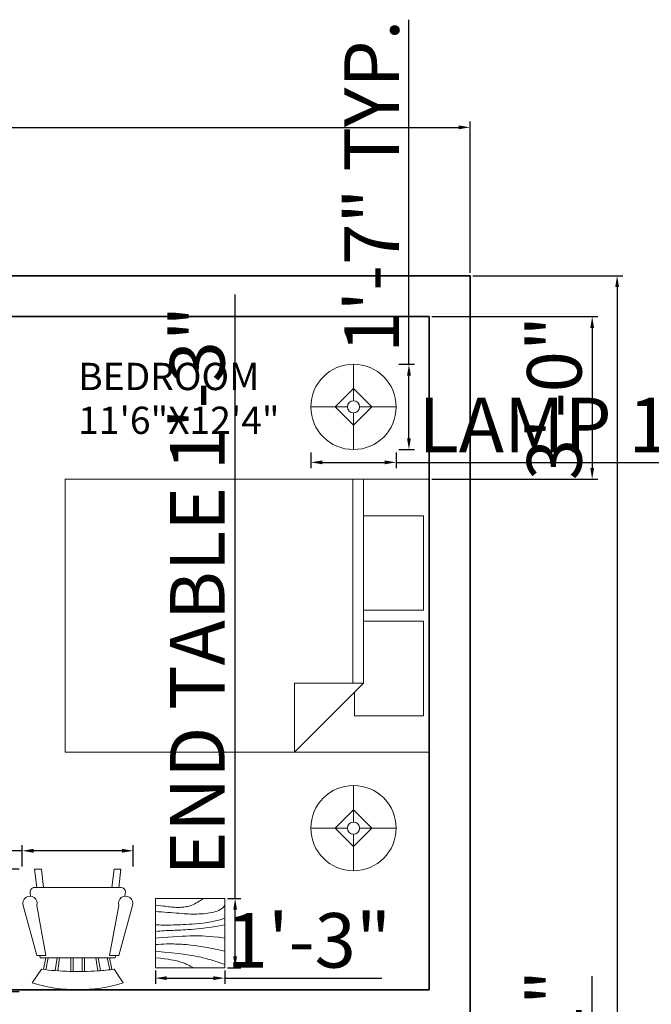
# Model space of a CAD drawing. Units: inches. Extents: x 2446 to 3341, y 462 to 1195.
# Tile 4 of 6: x 2746 to 2884, y 888 to 1104. Entities that reach past the tile are written whole.
import ezdxf

# ---------------------------------------------------------------- set-up
doc = ezdxf.new("R2010")
doc.units = ezdxf.units.IN
for name, color, linetype, lineweight in [('A-ANNO-DIMS', 2, 'Continuous', 18), ('A-AREA-IDEN', 7, 'Continuous', 18), ('A-FURN', 8, 'Continuous', 18), ('A-WALL', 7, 'Continuous', 35), ('C-PROP', 7, 'Continuous', 35)]:
    doc.layers.add(name, color=color, linetype=linetype, lineweight=lineweight)
doc.styles.get("Standard").update_dxf_attribs({"font": 'arial.ttf'})
doc.dimstyles.new('ISO-25', dxfattribs={"dimtxt": 12, "dimasz": 2.5, "dimexe": 1.25, "dimexo": 0.625, "dimtad": 1, "dimdec": 1, "dimlunit": 3, "dimtxsty": 'Standard', "dimcen": 2.5, "dimadec": 0, "dimazin": 0, "dimtfac": 1, "dimtdec": 1, "dimtmove": 0, "dimatfit": 3, "dimfxl": 1, "dimarcsym": 0})

# ---------------------------------------------------------------- blocks, each defined once
blk = doc.blocks.new('Bed - Queen')
for p, q in [((0, -80.00003), (0, 0)), ((0, 0), (59.99999, 0)), ((59.99999, 0), (59.99999, -80.00003)), ((7.99999, -1.2), (28.79998, -1.2)), ((7.99999, -14.4), (7.99999, -1.2)), ((28.79998, -1.2), (28.79998, -14.4)), ((31.19999, -1.2), (51.99999, -1.2)), ((31.19999, -14.4), (31.19999, -1.2)), ((51.99999, -1.2), (51.99999, -16.4)), ((0, -14.4), (44.8, -14.4)), ((59.99999, -29.6), (44.8, -14.4)), ((44.8, -14.4), (44.8, -29.6)), ((44.8, -16.8), (0, -16.8)), ((51.99999, -16.4), (46.79936, -16.4)), ((44.8, -29.6), (59.99999, -29.6)), ((59.99999, -80.00003), (0, -80.00003))]:
    blk.add_line(p, q)
blk = doc.blocks.new('Lamp - Table')
for p, q in [((0, 7), (0, 1)), ((0, 3), (-3, 0)), ((3, 0), (0, 3)), ((-1, 0), (-7, 0)), ((-3, 0), (0, -3)), ((0, -3), (3, 0)), ((1, 0), (7, 0)), ((0, -1), (0, -7))]:
    blk.add_line(p, q)
for radius in [7, 1]:
    blk.add_circle((0, 0), radius)
blk = doc.blocks.new('Chair - Rocking')
for p, q in [((-8, -4.5), (-10, -1.5)), ((8, -4.5), (10, -1.5)), ((-4.5, -7), (-4.96674, -4.19951)), ((-4, -7), (-4.40532, -4.16272)), ((-1.5, -4.05012), (-1.5, -7)), ((-1, -7), (-1, -4.05012)), ((1, -7), (1, -4.04655)), ((1.5, -4.05012), (1.5, -7)), ((4, -7), (4.40187, -4.18694)), ((4.5, -7), (4.96761, -4.19437)), ((-7.5, -4.5), (-7, -7)), ((-6.5, -7), (-7.02225, -4.43)), ((6.5, -7), (7, -4.4057)), ((7.5, -4.5), (7, -7)), ((-9, -7.5), (-12, -18.49999)), ((-7, -7.5), (-9, -7.5)), ((-9, -18.49999), (-7, -7.5)), ((-8.23428, -6.99939), (-8.3093, -7.47958)), ((-8.23041, -7), (8.23915, -7)), ((7, -7.5), (9, -7.5)), ((9, -18.49999), (7, -7.5)), ((8.31071, -7.48854), (8.23449, -7.00073)), ((9, -7.5), (12, -18.49999)), ((-10.36644, -20.64523), (-10.5, -21.49999)), ((10.5, -21.49999), (10.3575, -20.58798)), ((-9, -22.49999), (-9.5, -26.49999)), ((0, -22.49999), (-9.5, -22.49999)), ((-8, -26.49999), (-7.5, -22.49999)), ((0, -22.49999), (9.5, -22.49999)), ((8, -26.49999), (7.5, -22.49999)), ((9, -22.49999), (9.5, -26.49999)), ((-9.5, -26.49999), (-8, -26.49999)), ((9.5, -26.49999), (8, -26.49999))]:
    blk.add_line(p, q)
for centre, radius, start, end in [((0, -34.08333), 34.08333, 72.93847, 107.0615), ((0, -68.25004), 64.25, 93.92211, 97.15267), ((0, -68.25004), 64.25, 82.84733, 93.92211), ((-10.5, -18.99999), 1.58114, 161.5651, 18.43495), ((10.5, -18.99999), 1.58114, 161.5651, 18.43495), ((-9.5, -21.49999), 1, 180, 270), ((9.5, -21.49999), 1, 270, 0)]:
    blk.add_arc(centre, radius, start, end)
blk = doc.blocks.new('Table - Square Woodgrain 42 x 42 in.')
blk.add_line((0, -42), (42, -42))
for points in [[(0, -4), (1.704, -4.2172), (3.2358, -4.4188), (4.615, -4.604), (5.8615, -4.7721), (6.9951, -4.9224), (8.0357, -5.0541), (9.0031, -5.1667), (9.9171, -5.2594), (10.7951, -5.3316), (11.6445, -5.3836), (12.4702, -5.4157), (13.277, -5.4283), (14.0698, -5.4217), (14.8535, -5.3964), (15.6331, -5.3526), (16.4133, -5.2908), (17.1986, -5.2103), (17.9913, -5.1062), (18.793, -4.9727), (19.6056, -4.8038), (20.4307, -4.5937), (21.2701, -4.3365), (22.1256, -4.0262), (22.9989, -3.6571), (23.888, -3.2272), (24.7756, -2.7516), (25.6408, -2.2491), (26.4624, -1.7387), (27.2195, -1.2395), (27.891, -0.7703), (28.456, -0.3501), (28.8934, 0.002)], [(0, -42), (0, 0), (42, 0), (42, -42)], [(0, -8), (1.8203, -8.1001), (3.6741, -8.2149), (5.5411, -8.3408), (7.4011, -8.4741), (9.2339, -8.6112), (11.0193, -8.7484), (12.7371, -8.8821), (14.3671, -9.0086), (15.8954, -9.1246), (17.3337, -9.2278), (18.6997, -9.3159), (20.0116, -9.387), (21.2871, -9.4389), (22.5442, -9.4696), (23.8008, -9.477), (25.0749, -9.459), (26.3791, -9.4137), (27.7049, -9.3403), (29.0383, -9.2382), (30.3655, -9.1068), (31.6728, -8.9455), (32.9461, -8.7535), (34.1717, -8.5304), (35.3358, -8.2756), (36.4268, -7.9863), (37.443, -7.6521), (38.3849, -7.2603), (39.253, -6.7986), (40.048, -6.2542), (40.7705, -5.6147), (41.421, -4.8674), (42, -4)], [(42, -12), (39.1784, -12.8621), (36.4519, -13.5654), (33.8246, -14.1294), (31.3004, -14.5731), (28.8832, -14.9161), (26.577, -15.1775), (24.3858, -15.3768), (22.3136, -15.5332), (20.3622, -15.6632), (18.5254, -15.7718), (16.7947, -15.8612), (15.1618, -15.9338), (13.6183, -15.9916), (12.1558, -16.0369), (10.7659, -16.0718), (9.4403, -16.0987), (8.1703, -16.1191), (6.9461, -16.1325), (5.7577, -16.1377), (4.595, -16.1335), (3.4479, -16.1188), (2.3064, -16.0924), (1.1604, -16.0532), (0, -16)], [(42, -16), (37.6529, -16.7365), (33.8802, -17.329), (30.6179, -17.7961), (27.8015, -18.1561), (25.3668, -18.4275), (23.2497, -18.6288), (21.3859, -18.7785), (19.7111, -18.8949), (18.1693, -18.9939), (16.7375, -19.0795), (15.401, -19.1534), (14.1449, -19.217), (12.9544, -19.2717), (11.8148, -19.3191), (10.7113, -19.3606), (9.6291, -19.3976), (8.5534, -19.4323), (7.47, -19.4689), (6.3643, -19.5122), (5.222, -19.5672), (4.0288, -19.6386), (2.7703, -19.7313), (1.4321, -19.8501), (0, -20)], [(0, -24), (3.9243, -23.6805), (7.4766, -23.4138), (10.6891, -23.1954), (13.5943, -23.0205), (16.2247, -22.8847), (18.6125, -22.7832), (20.7903, -22.7116), (22.7903, -22.6651), (24.6563, -22.642), (26.4764, -22.6507), (28.35, -22.7024), (30.3766, -22.8084), (32.6555, -22.98), (35.2861, -23.2283), (38.3678, -23.5645), (42, -24)], [(42, -32), (37.392, -31.017), (33.4585, -30.2231), (30.1291, -29.5949), (27.3334, -29.109), (25.0009, -28.742), (23.0612, -28.4707), (21.4439, -28.2716), (20.0786, -28.1215), (18.8998, -28.0002), (17.8609, -27.9014), (16.9206, -27.8219), (16.0371, -27.7588), (15.1691, -27.709), (14.2748, -27.6693), (13.3128, -27.6368), (12.2415, -27.6083), (11.0295, -27.5824), (9.6867, -27.5643), (8.233, -27.5608), (6.6884, -27.5787), (5.0728, -27.6248), (3.4062, -27.7058), (1.7086, -27.8286), (0, -28)], [(0, -32), (5.4026, -32.5358), (9.9494, -33.019), (13.7424, -33.4553), (16.8834, -33.8505), (19.4743, -34.2106), (21.6171, -34.5413), (23.4136, -34.8486), (24.9657, -35.1382), (26.3614, -35.4156), (27.6332, -35.6841), (28.7995, -35.9467), (29.8788, -36.2064), (30.8897, -36.4661), (31.8507, -36.7288), (32.7802, -36.9973), (33.6968, -37.2747), (34.6175, -37.5635), (35.5531, -37.8651), (36.5128, -38.1805), (37.506, -38.5108), (38.5421, -38.8568), (39.6302, -39.2197), (40.7797, -39.6004), (42, -40)], [(0, -36), (3.0098, -36.2857), (5.5354, -36.5643), (7.6368, -36.8359), (9.374, -37.1009), (10.807, -37.3597), (11.9957, -37.6126), (13.0002, -37.8599), (13.8804, -38.102), (14.6874, -38.3393), (15.4365, -38.5729), (16.1338, -38.8041), (16.7858, -39.0341), (17.3987, -39.264), (17.9787, -39.4952), (18.5322, -39.7288), (19.0655, -39.9662), (19.5832, -40.2081), (20.0842, -40.4544), (20.5657, -40.7046), (21.0249, -40.9581), (21.459, -41.2144), (21.8653, -41.4731), (22.2409, -41.7335), (22.5831, -41.9951)]]:
    blk.add_lwpolyline(points)
blk = doc.blocks.new('*D17')
at = {"layer": 'A-ANNO-DIMS', "color": 0, "lineweight": -2, "transparency": 16777216}
for p, q in [((2544.62, 1048.59), (2544.62, 1081.85)), ((2547.12, 1080.6), (2842.12, 1080.6)), ((2844.62, 1048.59), (2844.62, 1081.85))]:
    blk.add_line(p, q, dxfattribs=at)
at = {"layer": 'A-ANNO-DIMS', "color": 0, "transparency": 16777216}
for points in [[(2547.12, 1081.02), (2547.12, 1080.18), (2544.62, 1080.6)], [(2842.12, 1081.02), (2842.12, 1080.18), (2844.62, 1080.6)]]:
    blk.add_solid(points, dxfattribs=at)
at = {"layer": 'Defpoints', "color": 0, "transparency": 16777216}
for p in [(2844.62, 1080.6), (2544.62, 1047.97), (2844.62, 1047.97)]:
    blk.add_point(p, dxfattribs=at)
at = {"layer": 'A-ANNO-DIMS', "color": 0, "transparency": 16777216, "insert": (2694.62, 1087.35), "char_height": 12, "attachment_point": 5}
blk.add_mtext("25'", dxfattribs=at)
blk = doc.blocks.new('*D18')
at = {"layer": 'A-ANNO-DIMS', "color": 0, "lineweight": -2, "transparency": 16777216}
for p, q in [((2845.24, 1047.97), (2878.2, 1047.97)), ((2876.95, 1045.47), (2876.95, 570.47)), ((2845.24, 567.97), (2878.2, 567.97))]:
    blk.add_line(p, q, dxfattribs=at)
at = {"layer": 'A-ANNO-DIMS', "color": 0, "transparency": 16777216}
for points in [[(2876.53, 1045.47), (2877.37, 1045.47), (2876.95, 1047.97)], [(2876.53, 570.47), (2877.37, 570.47), (2876.95, 567.97)]]:
    blk.add_solid(points, dxfattribs=at)
at = {"layer": 'Defpoints', "color": 0, "transparency": 16777216}
for p in [(2844.62, 1047.97), (2844.62, 567.97), (2876.95, 567.97)]:
    blk.add_point(p, dxfattribs=at)
at = {"layer": 'A-ANNO-DIMS', "color": 0, "transparency": 16777216, "insert": (2870.2, 807.97), "char_height": 12, "attachment_point": 5, "rotation": 90}
blk.add_mtext("40'", dxfattribs=at)
blk = doc.blocks.new('*D25')
at = {"layer": 'A-ANNO-DIMS', "color": 0, "lineweight": -2, "transparency": 16777216}
for p, q in [((2809.62, 1009.12), (2809.62, 1005.68)), ((2828.38, 1009.12), (2828.38, 1005.68)), ((2812.12, 1006.93), (2825.88, 1006.93)), ((2828.38, 1006.93), (2955.05, 1006.93))]:
    blk.add_line(p, q, dxfattribs=at)
at = {"layer": 'A-ANNO-DIMS', "color": 0, "transparency": 16777216}
for points in [[(2812.12, 1007.35), (2812.12, 1006.52), (2809.62, 1006.93)], [(2825.88, 1007.35), (2825.88, 1006.52), (2828.38, 1006.93)]]:
    blk.add_solid(points, dxfattribs=at)
at = {"layer": 'Defpoints', "color": 0, "transparency": 16777216}
for p in [(2809.62, 1009.75), (2828.38, 1009.75), (2828.38, 1006.93)]:
    blk.add_point(p, dxfattribs=at)
at = {"layer": 'A-ANNO-DIMS', "color": 0, "transparency": 16777216, "insert": (2892.96, 1013.59), "char_height": 12, "attachment_point": 5}
blk.add_mtext('LAMP 1\'-7" TYP.', dxfattribs=at)
blk = doc.blocks.new('*D26')
at = {"layer": 'A-ANNO-DIMS', "color": 0, "lineweight": -2, "transparency": 16777216}
for p, q in [((2831.19, 1028.51), (2831.19, 1104.27)), ((2829, 1028.51), (2832.44, 1028.51)), ((2831.19, 1012.25), (2831.19, 1026.01)), ((2829, 1009.75), (2832.44, 1009.75))]:
    blk.add_line(p, q, dxfattribs=at)
at = {"layer": 'A-ANNO-DIMS', "color": 0, "transparency": 16777216}
for points in [[(2830.77, 1026.01), (2831.61, 1026.01), (2831.19, 1028.51)], [(2830.77, 1012.25), (2831.61, 1012.25), (2831.19, 1009.75)]]:
    blk.add_solid(points, dxfattribs=at)
at = {"layer": 'Defpoints', "color": 0, "transparency": 16777216}
for p in [(2828.38, 1028.51), (2831.19, 1028.51), (2828.38, 1009.75)]:
    blk.add_point(p, dxfattribs=at)
at = {"layer": 'A-ANNO-DIMS', "color": 0, "transparency": 16777216, "insert": (2824.54, 1067.64), "char_height": 12, "attachment_point": 5, "rotation": 90}
blk.add_mtext('1\'-7" TYP.', dxfattribs=at)
blk = doc.blocks.new('*D33')
at = {"layer": 'A-ANNO-DIMS', "color": 0, "lineweight": -2, "transparency": 16777216}
for p, q in [((2745.53, 917.47), (2740.86, 917.47)), ((2742.11, 914.97), (2742.11, 892.97)), ((2745.53, 890.47), (2740.86, 890.47)), ((2742.11, 890.47), (2742.11, 737.82))]:
    blk.add_line(p, q, dxfattribs=at)
at = {"layer": 'A-ANNO-DIMS', "color": 0, "transparency": 16777216}
for points in [[(2741.69, 914.97), (2742.53, 914.97), (2742.11, 917.47)], [(2741.69, 892.97), (2742.53, 892.97), (2742.11, 890.47)]]:
    blk.add_solid(points, dxfattribs=at)
at = {"layer": 'Defpoints', "color": 0, "transparency": 16777216}
for p in [(2746.16, 917.47), (2742.11, 890.47), (2746.16, 890.47)]:
    blk.add_point(p, dxfattribs=at)
at = {"layer": 'A-ANNO-DIMS', "color": 0, "transparency": 16777216, "insert": (2735.27, 812.89), "char_height": 12, "attachment_point": 5, "rotation": 90}
blk.add_mtext('ROCKER 2\'-3" TYP.', dxfattribs=at)
blk = doc.blocks.new('*D34')
at = {"layer": 'A-ANNO-DIMS', "color": 0, "lineweight": -2, "transparency": 16777216}
for p, q in [((2746.16, 918.09), (2746.16, 922.77)), ((2770.59, 918.09), (2770.59, 922.77)), ((2746.16, 921.52), (2641.1, 921.52)), ((2768.09, 921.52), (2748.66, 921.52))]:
    blk.add_line(p, q, dxfattribs=at)
at = {"layer": 'A-ANNO-DIMS', "color": 0, "transparency": 16777216}
for points in [[(2748.66, 921.94), (2748.66, 921.1), (2746.16, 921.52)], [(2768.09, 921.94), (2768.09, 921.1), (2770.59, 921.52)]]:
    blk.add_solid(points, dxfattribs=at)
at = {"layer": 'Defpoints', "color": 0, "transparency": 16777216}
for p in [(2746.16, 921.52), (2746.16, 917.47), (2770.59, 917.47)]:
    blk.add_point(p, dxfattribs=at)
at = {"layer": 'A-ANNO-DIMS', "color": 0, "transparency": 16777216, "insert": (2692.38, 928.35), "char_height": 12, "attachment_point": 5}
blk.add_mtext('2\'-0 1/2" TYP.', dxfattribs=at)
blk = doc.blocks.new('*D37')
at = {"layer": 'A-ANNO-DIMS', "color": 0, "lineweight": -2, "transparency": 16777216}
for p, q in [((2792.98, 911.05), (2792.98, 1043.88)), ((2791.32, 911.05), (2794.23, 911.05)), ((2792.98, 898.3), (2792.98, 908.55)), ((2791.32, 895.8), (2794.23, 895.8))]:
    blk.add_line(p, q, dxfattribs=at)
at = {"layer": 'A-ANNO-DIMS', "color": 0, "transparency": 16777216}
for points in [[(2792.56, 908.55), (2793.39, 908.55), (2792.98, 911.05)], [(2792.56, 898.3), (2793.39, 898.3), (2792.98, 895.8)]]:
    blk.add_solid(points, dxfattribs=at)
at = {"layer": 'Defpoints', "color": 0, "transparency": 16777216}
for p in [(2790.69, 911.05), (2792.98, 911.05), (2790.69, 895.8)]:
    blk.add_point(p, dxfattribs=at)
at = {"layer": 'A-ANNO-DIMS', "color": 0, "transparency": 16777216, "insert": (2786.22, 978.71), "char_height": 12, "attachment_point": 5, "rotation": 90}
blk.add_mtext('END TABLE 1\'-3"', dxfattribs=at)
blk = doc.blocks.new('*D38')
at = {"layer": 'A-ANNO-DIMS', "color": 0, "lineweight": -2, "transparency": 16777216}
for p, q in [((2775.45, 895.18), (2775.45, 892.27)), ((2790.69, 895.18), (2790.69, 892.27)), ((2777.95, 893.52), (2788.19, 893.52)), ((2790.69, 893.52), (2825.21, 893.52))]:
    blk.add_line(p, q, dxfattribs=at)
at = {"layer": 'A-ANNO-DIMS', "color": 0, "transparency": 16777216}
for points in [[(2777.95, 893.93), (2777.95, 893.1), (2775.45, 893.52)], [(2788.19, 893.93), (2788.19, 893.1), (2790.69, 893.52)]]:
    blk.add_solid(points, dxfattribs=at)
at = {"layer": 'Defpoints', "color": 0, "transparency": 16777216}
for p in [(2775.45, 895.8), (2790.69, 895.8), (2790.69, 893.52)]:
    blk.add_point(p, dxfattribs=at)
at = {"layer": 'A-ANNO-DIMS', "color": 0, "transparency": 16777216, "insert": (2809.2, 900.27), "char_height": 12, "attachment_point": 5}
blk.add_mtext('1\'-3"', dxfattribs=at)
blk = doc.blocks.new('*D62')
at = {"layer": 'A-ANNO-DIMS', "color": 0, "lineweight": -2, "transparency": 16777216}
for p, q in [((2871.47, 848.97), (2871.47, 893.94)), ((2782.24, 848.97), (2872.72, 848.97)), ((2871.47, 840.47), (2871.47, 846.47)), ((2782.24, 837.97), (2872.72, 837.97))]:
    blk.add_line(p, q, dxfattribs=at)
at = {"layer": 'A-ANNO-DIMS', "color": 0, "transparency": 16777216}
for points in [[(2871.05, 846.47), (2871.88, 846.47), (2871.47, 848.97)], [(2871.05, 840.47), (2871.88, 840.47), (2871.47, 837.97)]]:
    blk.add_solid(points, dxfattribs=at)
at = {"layer": 'Defpoints', "color": 0, "transparency": 16777216}
for p in [(2781.62, 848.97), (2871.47, 848.97), (2781.62, 837.97)]:
    blk.add_point(p, dxfattribs=at)
at = {"layer": 'A-ANNO-DIMS', "color": 0, "transparency": 16777216, "insert": (2864.71, 872.71), "char_height": 12, "attachment_point": 5, "rotation": 90}
blk.add_mtext('0\'-11"', dxfattribs=at)
blk = doc.blocks.new('*D75')
at = {"layer": 'A-ANNO-DIMS', "color": 0, "lineweight": -2, "transparency": 16777216}
for p, q in [((2836.24, 1038.97), (2872.72, 1038.97)), ((2871.47, 1036.47), (2871.47, 1005.7)), ((2836.24, 1003.2), (2872.72, 1003.2))]:
    blk.add_line(p, q, dxfattribs=at)
at = {"layer": 'A-ANNO-DIMS', "color": 0, "transparency": 16777216}
for points in [[(2871.05, 1036.47), (2871.88, 1036.47), (2871.47, 1038.97)], [(2871.05, 1005.7), (2871.88, 1005.7), (2871.47, 1003.2)]]:
    blk.add_solid(points, dxfattribs=at)
at = {"layer": 'Defpoints', "color": 0, "transparency": 16777216}
for p in [(2835.62, 1038.97), (2835.62, 1003.2), (2871.47, 1003.2)]:
    blk.add_point(p, dxfattribs=at)
at = {"layer": 'A-ANNO-DIMS', "color": 0, "transparency": 16777216, "insert": (2864.71, 1021.08), "char_height": 12, "attachment_point": 5, "rotation": 90}
blk.add_mtext('3\'-0"', dxfattribs=at)

msp = doc.modelspace()

# ---------------------------------------------------------------- linework, layer by layer
at = {"layer": 'A-WALL'}
for p, q in [((2835.62, 1038.97), (2699.62, 1038.97)), ((2835.62, 890.97), (2835.62, 1038.97)), ((2835.62, 890.97), (2699.62, 890.97))]:
    msp.add_line(p, q, dxfattribs=at)
at = {"layer": 'C-PROP'}
msp.add_lwpolyline([(2544.62, 567.97), (2844.62, 567.97), (2844.62, 1047.97), (2544.62, 1047.97)], close=True, dxfattribs=at)

# ---------------------------------------------------------------- block references
at = {"layer": 'A-FURN'}
for name, p, xscale, yscale, zscale in [('Lamp - Table', (2819, 1019.13), 1.339901149487936, 1.339901149487936, 1.339901149487936), ('Lamp - Table', (2819, 926.5), 1.339901149487936, 1.339901149487936, 1.339901149487936), ('Table - Square Woodgrain 42 x 42 in.', (2775.45, 911.04), 0.3629084931323049, 0.3629084931323049, 0.3629084931323049)]:
    msp.add_blockref(name, p, dxfattribs=dict(at, xscale=xscale, yscale=yscale, zscale=zscale))
for name, p, rotation in [('Bed - Queen', (2835.62, 1003.2), 270), ('Chair - Rocking', (2758.38, 890.97), 180)]:
    msp.add_blockref(name, p, dxfattribs=dict(at, rotation=rotation))

# ---------------------------------------------------------------- texts
at = {"layer": 'A-AREA-IDEN'}
for s, p in [('BEDROOM', (2758.48, 1022.82)), ('11\'6"X12\'4"', (2758.48, 1013.18))]:
    msp.add_text(s, height=6, dxfattribs=at).set_placement(p)

# ---------------------------------------------------------------- dimensions: what is measured, and where the dimension line sits
at = {"layer": 'A-ANNO-DIMS'}
for base, p1, p2, angle, text, picture, middle in [((2831.19, 1028.51), (2828.38, 1009.75), (2828.38, 1028.51), 90, '<> TYP.', '*D26', (2824.54, 1067.64)), ((2792.9765, 911.0456), (2790.6901, 895.8027), (2790.6901, 911.0456), 90, 'END TABLE <>', '*D37', (2786.2205, 978.7135)), ((2746.16, 921.52), (2770.59, 917.47), (2746.16, 917.47), 180, '<> TYP.', '*D34', (2692.38, 928.35)), ((2742.11, 890.47), (2746.16, 917.47), (2746.16, 890.47), 270, 'ROCKER <> TYP.', '*D33', (2735.27, 812.89))]:
    dim = msp.add_linear_dim(base=base, p1=p1, p2=p2, angle=angle, text=text, dimstyle='ISO-25', override={"dimdec": 1, "dimlfac": 1, "dimrnd": 0, "dimzin": 1, "dimdsep": 46, "dimlunit": 4, "dimfrac": 2}, dxfattribs=at)
    dim.commit()
    dim.dimension.update_dxf_attribs({"geometry": picture, "text_midpoint": middle})
for base, p1, p2, override, picture, middle in [((2844.62, 1080.6), (2544.62, 1047.97), (2844.62, 1047.97), {"dimclrd": 0, "dimclre": 0, "dimclrt": 0}, '*D17', (2694.62, 1087.35)), ((2790.69, 893.52), (2775.45, 895.8), (2790.69, 895.8), {"dimdec": 1, "dimlfac": 1, "dimrnd": 0, "dimzin": 1, "dimdsep": 46, "dimlunit": 4, "dimfrac": 2}, '*D38', (2809.2, 900.27))]:
    dim = msp.add_linear_dim(base=base, p1=p1, p2=p2, dimstyle='ISO-25', override=override, dxfattribs=at)
    dim.commit()
    dim.dimension.update_dxf_attribs({"geometry": picture, "text_midpoint": middle})
for base, p1, p2, override, picture, middle in [((2876.95, 567.97), (2844.62, 1047.97), (2844.62, 567.97), {"dimclrd": 0, "dimclre": 0, "dimclrt": 0}, '*D18', (2870.2, 807.97)), ((2871.47, 1003.2), (2835.62, 1038.97), (2835.62, 1003.2), {"dimdec": 1, "dimlfac": 1, "dimrnd": 0, "dimzin": 1, "dimdsep": 46, "dimlunit": 4, "dimfrac": 2}, '*D75', (2864.71, 1021.08)), ((2871.47, 848.97), (2781.62, 837.97), (2781.62, 848.97), {"dimdec": 1, "dimlfac": 1, "dimrnd": 0, "dimzin": 1, "dimdsep": 46, "dimlunit": 4, "dimfrac": 2}, '*D62', (2864.71, 872.71))]:
    dim = msp.add_linear_dim(base=base, p1=p1, p2=p2, angle=90, dimstyle='ISO-25', override=override, dxfattribs=at)
    dim.commit()
    dim.dimension.update_dxf_attribs({"geometry": picture, "text_midpoint": middle})
dim = msp.add_linear_dim(base=(2828.38, 1006.93), p1=(2809.62, 1009.75), p2=(2828.38, 1009.75), text='LAMP <> TYP.', dimstyle='ISO-25', override={"dimdec": 1, "dimlfac": 1, "dimrnd": 0, "dimzin": 1, "dimdsep": 46, "dimlunit": 4, "dimfrac": 2}, dxfattribs=at)
dim.commit()
dim.dimension.update_dxf_attribs({"geometry": '*D25', "text_midpoint": (2892.96, 1013.59)})

doc.saveas('drawing.dxf')
